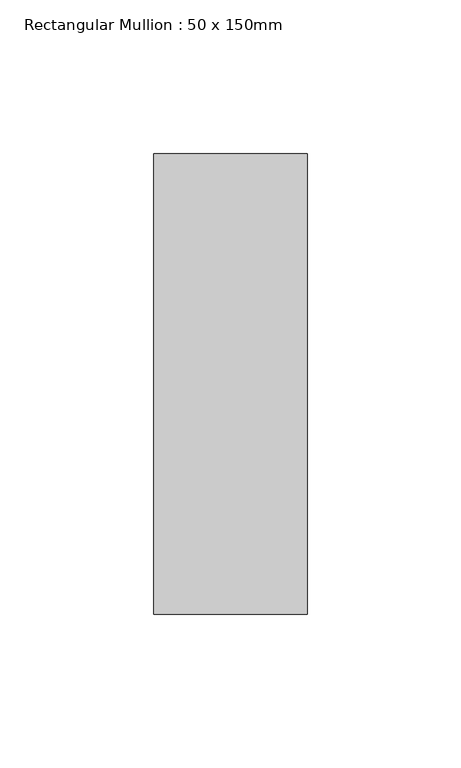
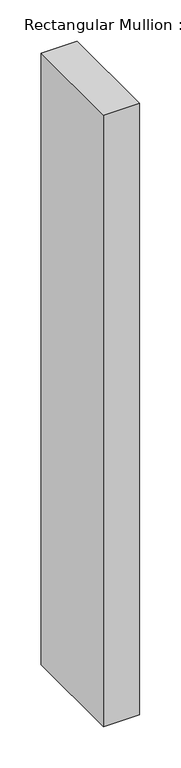
"""IFC4 building model written with IfcOpenShell, lengths in millimetres: member geometry, Rectangular Mullion : 50 x 150mm."""

from ifc_helpers import new_model, si_unit, frame, origin, place, context, project, spatial, polyline, outline, extrude, source, transform, mapped, element, save


def rectangular_mullion_50_x_150mm_35d6a770(model_context):
    return source(origin(), model_context, "Body", "SweptSolid", [
        extrude(outline(polyline([(0.0, 75.0), (0.0, -75.0), (-50.0, -75.0), (-50.0, 75.0), (0.0, 75.0)])), frame((0.0, 0.0, -900.0), z_axis=(0.0, 0.0, 1.0), x_axis=(1.0, 0.0, 0.0)), (0.0, 0.0, 1.0), 900.0),
    ])


if __name__ == "__main__":
    model = new_model("IFC4")
    model_context = context("Model", 3, world=origin())
    ifc_project = project(units=[si_unit("LENGTHUNIT", "METRE", prefix="MILLI")], contexts=[model_context])
    site = spatial("IfcSite", under=ifc_project)
    building = spatial("IfcBuilding", under=site)
    placement = place(None, origin())
    rectangular_mullion_50_x_150mm_shape = rectangular_mullion_50_x_150mm_35d6a770(model_context)
    element("IfcMember", 1, ObjectType="Rectangular Mullion : 50 x 150mm", at=placement, inside=building, context=model_context, shape_type="MappedRepresentation", body=[
        mapped(rectangular_mullion_50_x_150mm_shape, transform((0.0, 0.0, 0.0), x_axis=(1.0, 0.0, 0.0), y_axis=(0.0, 1.0, 0.0), z_axis=(0.0, 0.0, 1.0))),
    ])
    save(model, "model.ifc")

# Revit data of these elements
# Type "Rectangular Mullion : 50 x 150mm"
#   built-in parameter 1007304 = 0.492126 (stored number, unit not read)
#   built-in parameter 1007301 = 0.082021 (stored number, unit not read)
#   built-in parameter 1007300 = 0.082021 (stored number, unit not read)
# Element 1 (IfcMember, "Rectangular Mullion : 50 x 150mm")
#   Materials on its faces: "Aluminium"
# Materials
#   "Aluminium": class "Metal", colour RGB 247 247 247, transparency 0, Description = "Aluminium 6061", Cost = 0
